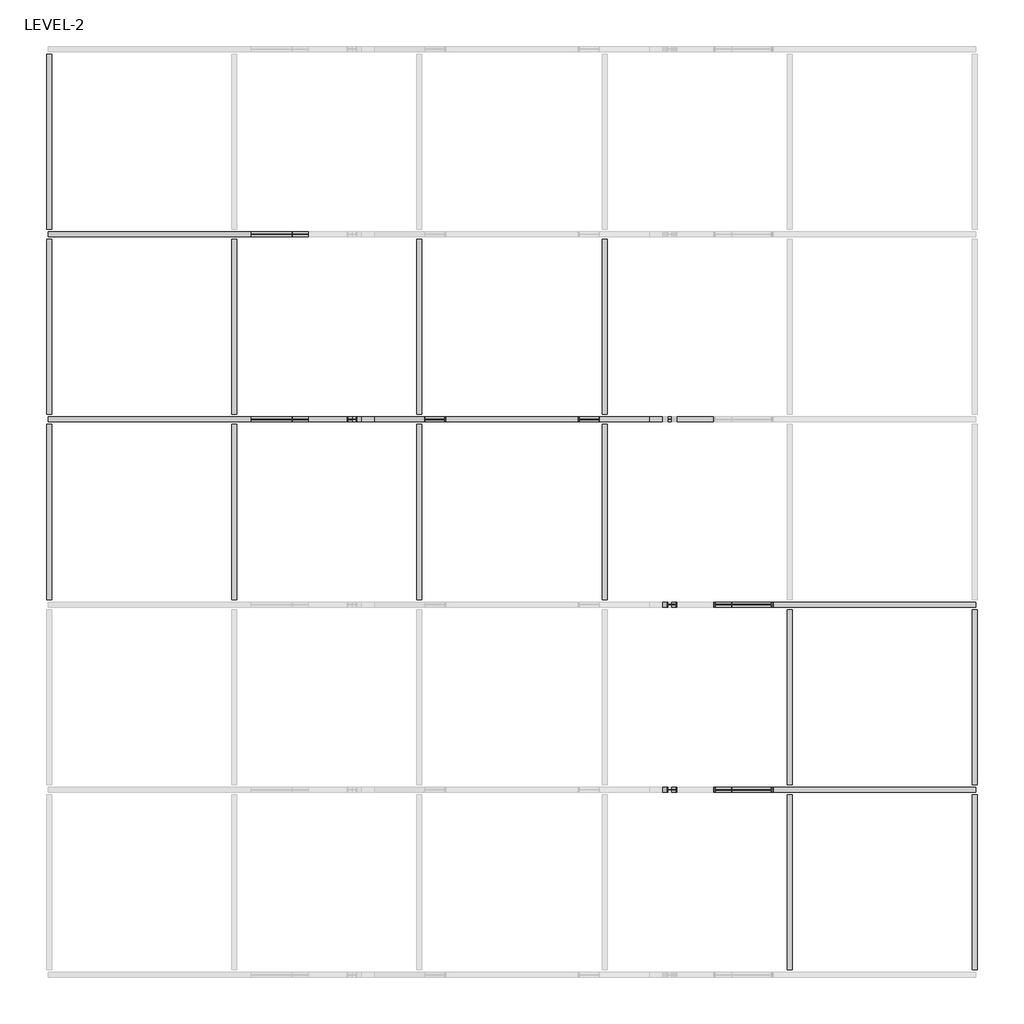
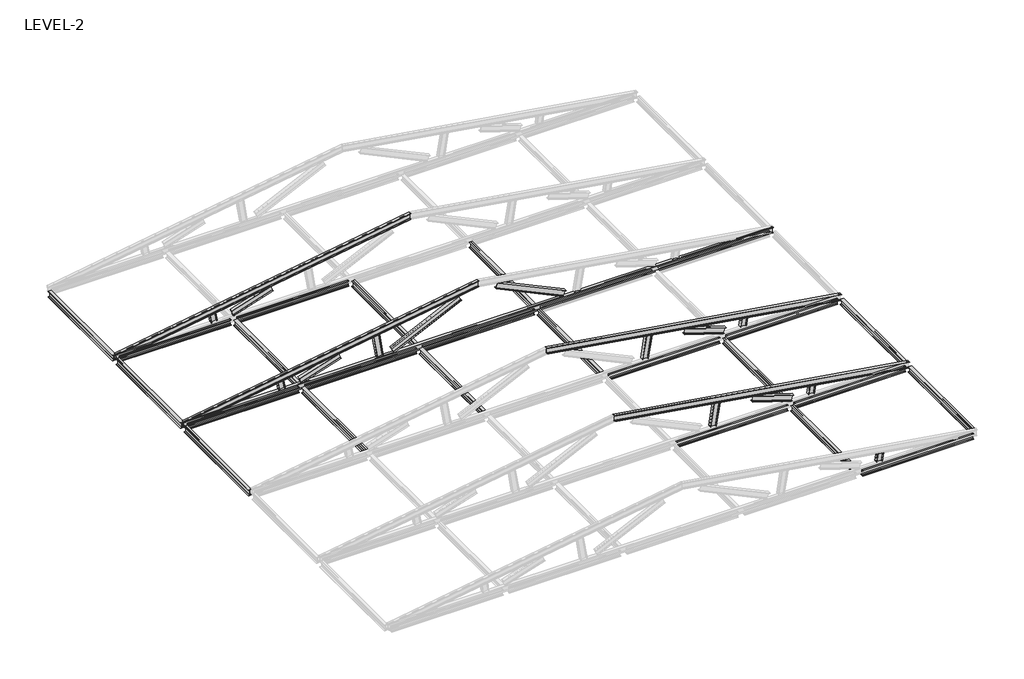
# One storey, part 2 of 3: 42 beams.
"""IFC4 building model written with IfcOpenShell, lengths in millimetres."""

from ifc_helpers import new_model, si_unit, frame, origin, place, context, project, spatial, polyline, circle_curve, ellipse_curve, transform, mapped, element, save
from ifc_brep_helpers import plane_surface, revolved_surface, advanced_brep
from components import ub_universal_beams_ub305x165x40_616d6e4e, ub_universal_beams_ub305x165x40_3f70edd5, ub_universal_beams_ub305x165x40_c9eec61f, ub_universal_beams_ub305x165x40_c956ba20, ub_universal_beams_ub305x165x40_f58164a9, ub_universal_beams_ub305x165x40_ef0a91e2, ub_universal_beams_ub305x165x40_83ed4f69, ub_universal_beams_ub305x165x40_46a3dc55, ub_universal_beams_ub305x165x40_0b6a72e4, ub_universal_beams_ub305x165x40_63d5ebb1, ub_universal_beams_ub305x165x40_05d28e63

model = new_model("IFC4")

# Units and contexts
model_context = context("Model", 3, world=origin())
ifc_project = project(units=[si_unit("LENGTHUNIT", "METRE", prefix="MILLI")], contexts=[model_context])

# Site, building, storey
site = spatial("IfcSite", under=ifc_project)
building = spatial("IfcBuilding", under=site)
storey = spatial("IfcBuildingStorey", under=building, Name="LEVEL-2", Elevation=4267.0)

# Beams
placement = place(None, origin())
element("IfcBeam", 1, ObjectType="UB-Universal Beams : UB305x165x40", at=placement, inside=storey, context=model_context, shape_type="AdvancedBrep", body=[
    advanced_brep(
    [(11917.6451312, -8149.9765895, 4127.2241081), (11917.6451312, -8220.5765895, 4127.2241081), (11919.0296431, -8229.4765895, 4136.0157591), (11960.2849884, -8229.4765895, 4397.9872012), (11961.6695003, -8220.5765895, 4406.7788522), (11961.6695003, -8149.9765895, 4406.7788522), (11963.2562444, -8149.9765895, 4416.8546768), (11963.2562444, -8314.9765895, 4416.8546768), (11961.6695003, -8314.9765895, 4406.7788522), (11961.6695003, -8244.3765895, 4406.7788522), (11960.2849884, -8235.4765895, 4397.9872012), (11919.0296431, -8235.4765895, 4136.0157591), (11917.6451312, -8244.3765895, 4127.2241081), (11917.6451312, -8314.9765895, 4127.2241081), (11916.0583871, -8314.9765895, 4117.1482834), (11916.0583871, -8149.9765895, 4117.1482834), (-3300.3332854, -8149.9765895, 6523.7561422), (-3300.3332854, -8220.5765895, 6523.7561422), (-3300.3332854, -8229.4765895, 6532.7658266), (-3300.3332854, -8229.4765895, 6801.2341734), (-3300.3332854, -8220.5765895, 6810.2438578), (-3300.3332854, -8149.9765895, 6810.2438578), (-3300.3332854, -8149.9765895, 6820.5695634), (-3300.3332854, -8314.9765895, 6820.5695634), (-3300.3332854, -8314.9765895, 6810.2438578), (-3300.3332854, -8244.3765895, 6810.2438578), (-3300.3332854, -8235.4765895, 6801.2341734), (-3300.3332854, -8235.4765895, 6532.7658266), (-3300.3332854, -8244.3765895, 6523.7561422), (-3300.3332854, -8314.9765895, 6523.7561422), (-3300.3332854, -8314.9765895, 6513.4304366), (-3300.3332854, -8149.9765895, 6513.4304366)],
    [
        (0, 1),
        (1, 2, circle_curve(frame((11919.0296431, -8220.5765895, 4136.0157591), z_axis=(-0.9878259507117182, 0.0, 0.1555631418443652), x_axis=(0.0, -1.0, 0.0)), 8.9)),
        (2, 3),
        (3, 4, circle_curve(frame((11960.2849884, -8220.5765895, 4397.9872012), z_axis=(-0.9878259507117182, 0.0, 0.1555631418443652), x_axis=(0.0, -1.0, 0.0)), 8.9)),
        (4, 5),
        (5, 6),
        (6, 7),
        (7, 8),
        (8, 9),
        (9, 10, circle_curve(frame((11960.2849884, -8244.3765895, 4397.9872012), z_axis=(-0.9878259507117182, 0.0, 0.1555631418443652), x_axis=(0.0, -1.0, 0.0)), 8.9)),
        (10, 11),
        (11, 12, circle_curve(frame((11919.0296431, -8244.3765895, 4136.0157591), z_axis=(-0.9878259507117182, 0.0, 0.1555631418443652), x_axis=(0.0, -1.0, 0.0)), 8.9)),
        (12, 13),
        (13, 14),
        (14, 15),
        (15, 0),
        (0, 16),
        (16, 17),
        (17, 1),
        (17, 18, ellipse_curve(frame((-3300.3332854, -8220.5765895, 6532.7658266), z_axis=(-1.0, 0.0, 0.0), x_axis=(0.0, 0.0, 1.0)), 9.0096843, 8.9)),
        (18, 2),
        (18, 19),
        (19, 3),
        (19, 20, ellipse_curve(frame((-3300.3332854, -8220.5765895, 6801.2341734), z_axis=(-1.0, 0.0, 0.0), x_axis=(0.0, 0.0, 1.0)), 9.0096843, 8.9)),
        (20, 4),
        (20, 21),
        (21, 5),
        (21, 22),
        (22, 6),
        (22, 23),
        (23, 7),
        (23, 24),
        (24, 8),
        (24, 25),
        (25, 9),
        (25, 26, ellipse_curve(frame((-3300.3332854, -8244.3765895, 6801.2341734), z_axis=(-1.0, 0.0, 0.0), x_axis=(0.0, 0.0, 1.0)), 9.0096843, 8.9)),
        (26, 10),
        (26, 27),
        (27, 11),
        (27, 28, ellipse_curve(frame((-3300.3332854, -8244.3765895, 6532.7658266), z_axis=(-1.0, 0.0, 0.0), x_axis=(0.0, 0.0, 1.0)), 9.0096843, 8.9)),
        (28, 12),
        (28, 29),
        (29, 13),
        (29, 30),
        (30, 14),
        (30, 31),
        (31, 15),
        (31, 16),
    ],
    [
        plane_surface(frame((11939.6573157, -8232.4765895, 4267.0014801), z_axis=(0.9878259507117182, 0.0, -0.1555631418443652), x_axis=(0.1555631418443652, 0.0, 0.9878259507117182))),
        plane_surface(frame((11917.6451312, -8149.9765895, 4127.2241081), z_axis=(0.1555631418443652, 0.0, 0.9878259507117182), x_axis=(-0.9878259507117182, 0.0, 0.1555631418443652))),
        revolved_surface(polyline([(-3301.7177973591024, -8229.4765895, 6532.983859959702), (11919.029643166847, -8229.4765895, 4136.015759089472)]), (11919.0296431, -8220.5765895, 4136.0157591), (-0.9878259507117182, 0.0, 0.1555631418443652)),
        plane_surface(frame((11919.0296431, -8229.4765895, 4136.0157591), z_axis=(0.0, 1.0, 0.0), x_axis=(-0.9878259507117182, 0.0, 0.1555631418443652))),
        revolved_surface(polyline([(-3301.717797363457, -8229.4765895, 6801.452206832042), (11960.2849884, -8229.4765895, 4397.9872012)]), (11960.2849884, -8220.5765895, 4397.9872012), (-0.9878259507117182, 0.0, 0.1555631418443652)),
        plane_surface(frame((11961.6695003, -8220.5765895, 4406.7788522), z_axis=(-0.1555631418443652, 0.0, -0.9878259507117182), x_axis=(-0.9878259507117182, 0.0, 0.1555631418443652))),
        plane_surface(frame((11961.6695003, -8149.9765895, 4406.7788522), z_axis=(0.0, 1.0, 0.0), x_axis=(-0.9878259507117182, 0.0, 0.1555631418443652))),
        plane_surface(frame((11963.2562444, -8149.9765895, 4416.8546768), z_axis=(0.1555631418443652, 0.0, 0.9878259507117182), x_axis=(-0.9878259507117182, 0.0, 0.1555631418443652))),
        plane_surface(frame((11963.2562444, -8314.9765895, 4416.8546768), z_axis=(0.0, -1.0, 0.0), x_axis=(-0.9878259507117182, 0.0, 0.1555631418443652))),
        plane_surface(frame((11961.6695003, -8314.9765895, 4406.7788522), z_axis=(-0.1555631418443652, 0.0, -0.9878259507117182), x_axis=(-0.9878259507117182, 0.0, 0.1555631418443652))),
        revolved_surface(polyline([(-3301.717797363457, -8253.2765895, 6801.452206832042), (11960.2849884, -8253.2765895, 4397.9872012)]), (11960.2849884, -8244.3765895, 4397.9872012), (-0.9878259507117182, 0.0, 0.1555631418443652)),
        plane_surface(frame((11960.2849884, -8235.4765895, 4397.9872012), z_axis=(0.0, -1.0, 0.0), x_axis=(-0.9878259507117182, 0.0, 0.1555631418443652))),
        revolved_surface(polyline([(-3301.7177973591024, -8253.2765895, 6532.983859959702), (11919.029643166847, -8253.2765895, 4136.015759089472)]), (11919.0296431, -8244.3765895, 4136.0157591), (-0.9878259507117182, 0.0, 0.1555631418443652)),
        plane_surface(frame((11917.6451312, -8244.3765895, 4127.2241081), z_axis=(0.1555631418443652, 0.0, 0.9878259507117182), x_axis=(-0.9878259507117182, 0.0, 0.1555631418443652))),
        plane_surface(frame((11917.6451312, -8314.9765895, 4127.2241081), z_axis=(0.0, -1.0, 0.0), x_axis=(-0.9878259507117182, 0.0, 0.1555631418443652))),
        plane_surface(frame((11916.0583871, -8314.9765895, 4117.1482834), z_axis=(-0.1555631418443652, 0.0, -0.9878259507117182), x_axis=(-0.9878259507117182, 0.0, 0.1555631418443652))),
        plane_surface(frame((11916.0583871, -8149.9765895, 4117.1482834), z_axis=(0.0, 1.0, 0.0), x_axis=(-0.9878259507117182, 0.0, 0.1555631418443652))),
        plane_surface(frame((-3300.3332854, -8232.4765895, 6820.5695634), z_axis=(-1.0, 0.0, 0.0), x_axis=(0.0, 1.0, 0.0))),
    ],
    [
        (0, [[1, 2, 3, 4, 5, 6, 7, 8, 9, 10, 11, 12, 13, 14, 15, 16]]),
        (1, [[-1, 17, 18, 19]]),
        (2, [[-2, -19, 20, 21]]),
        (3, [[-3, -21, 22, 23]]),
        (4, [[-4, -23, 24, 25]]),
        (5, [[-5, -25, 26, 27]]),
        (6, [[-6, -27, 28, 29]]),
        (7, [[-7, -29, 30, 31]]),
        (8, [[-8, -31, 32, 33]]),
        (9, [[-9, -33, 34, 35]]),
        (10, [[-10, -35, 36, 37]]),
        (11, [[-11, -37, 38, 39]]),
        (12, [[-12, -39, 40, 41]]),
        (13, [[-13, -41, 42, 43]]),
        (14, [[-14, -43, 44, 45]]),
        (15, [[-15, -45, 46, 47]]),
        (16, [[-16, -47, 48, -17]]),
        (17, [[-48, -46, -44, -42, -40, -38, -36, -34, -32, -30, -28, -26, -24, -22, -20, -18]]),
    ],
),
])
element("IfcBeam", 2, ObjectType="UB-Universal Beams : UB305x165x40", at=placement, inside=storey, context=model_context, shape_type="AdvancedBrep", body=[
    advanced_brep(
    [(11917.6451312, -2053.9765895, 4127.2241081), (11917.6451312, -2124.5765895, 4127.2241081), (11919.0296431, -2133.4765895, 4136.0157591), (11960.2849884, -2133.4765895, 4397.9872012), (11961.6695003, -2124.5765895, 4406.7788522), (11961.6695003, -2053.9765895, 4406.7788522), (11963.2562444, -2053.9765895, 4416.8546768), (11963.2562444, -2218.9765895, 4416.8546768), (11961.6695003, -2218.9765895, 4406.7788522), (11961.6695003, -2148.3765895, 4406.7788522), (11960.2849884, -2139.4765895, 4397.9872012), (11919.0296431, -2139.4765895, 4136.0157591), (11917.6451312, -2148.3765895, 4127.2241081), (11917.6451312, -2218.9765895, 4127.2241081), (11916.0583871, -2218.9765895, 4117.1482834), (11916.0583871, -2053.9765895, 4117.1482834), (-3300.3332854, -2053.9765895, 6523.7561422), (-3300.3332854, -2124.5765895, 6523.7561422), (-3300.3332854, -2133.4765895, 6532.7658266), (-3300.3332854, -2133.4765895, 6801.2341734), (-3300.3332854, -2124.5765895, 6810.2438578), (-3300.3332854, -2053.9765895, 6810.2438578), (-3300.3332854, -2053.9765895, 6820.5695634), (-3300.3332854, -2218.9765895, 6820.5695634), (-3300.3332854, -2218.9765895, 6810.2438578), (-3300.3332854, -2148.3765895, 6810.2438578), (-3300.3332854, -2139.4765895, 6801.2341734), (-3300.3332854, -2139.4765895, 6532.7658266), (-3300.3332854, -2148.3765895, 6523.7561422), (-3300.3332854, -2218.9765895, 6523.7561422), (-3300.3332854, -2218.9765895, 6513.4304366), (-3300.3332854, -2053.9765895, 6513.4304366)],
    [
        (0, 1),
        (1, 2, circle_curve(frame((11919.0296431, -2124.5765895, 4136.0157591), z_axis=(-0.9878259507117182, 0.0, 0.1555631418443652), x_axis=(0.0, -1.0, 0.0)), 8.9)),
        (2, 3),
        (3, 4, circle_curve(frame((11960.2849884, -2124.5765895, 4397.9872012), z_axis=(-0.9878259507117182, 0.0, 0.1555631418443652), x_axis=(0.0, -1.0, 0.0)), 8.9)),
        (4, 5),
        (5, 6),
        (6, 7),
        (7, 8),
        (8, 9),
        (9, 10, circle_curve(frame((11960.2849884, -2148.3765895, 4397.9872012), z_axis=(-0.9878259507117182, 0.0, 0.1555631418443652), x_axis=(0.0, -1.0, 0.0)), 8.9)),
        (10, 11),
        (11, 12, circle_curve(frame((11919.0296431, -2148.3765895, 4136.0157591), z_axis=(-0.9878259507117182, 0.0, 0.1555631418443652), x_axis=(0.0, -1.0, 0.0)), 8.9)),
        (12, 13),
        (13, 14),
        (14, 15),
        (15, 0),
        (0, 16),
        (16, 17),
        (17, 1),
        (17, 18, ellipse_curve(frame((-3300.3332854, -2124.5765895, 6532.7658266), z_axis=(-1.0, 0.0, 0.0), x_axis=(0.0, 0.0, 1.0)), 9.0096843, 8.9)),
        (18, 2),
        (18, 19),
        (19, 3),
        (19, 20, ellipse_curve(frame((-3300.3332854, -2124.5765895, 6801.2341734), z_axis=(-1.0, 0.0, 0.0), x_axis=(0.0, 0.0, 1.0)), 9.0096843, 8.9)),
        (20, 4),
        (20, 21),
        (21, 5),
        (21, 22),
        (22, 6),
        (22, 23),
        (23, 7),
        (23, 24),
        (24, 8),
        (24, 25),
        (25, 9),
        (25, 26, ellipse_curve(frame((-3300.3332854, -2148.3765895, 6801.2341734), z_axis=(-1.0, 0.0, 0.0), x_axis=(0.0, 0.0, 1.0)), 9.0096843, 8.9)),
        (26, 10),
        (26, 27),
        (27, 11),
        (27, 28, ellipse_curve(frame((-3300.3332854, -2148.3765895, 6532.7658266), z_axis=(-1.0, 0.0, 0.0), x_axis=(0.0, 0.0, 1.0)), 9.0096843, 8.9)),
        (28, 12),
        (28, 29),
        (29, 13),
        (29, 30),
        (30, 14),
        (30, 31),
        (31, 15),
        (31, 16),
    ],
    [
        plane_surface(frame((11939.6573157, -2136.4765895, 4267.0014801), z_axis=(0.9878259507117182, 0.0, -0.1555631418443652), x_axis=(0.1555631418443652, 0.0, 0.9878259507117182))),
        plane_surface(frame((11917.6451312, -2053.9765895, 4127.2241081), z_axis=(0.1555631418443652, 0.0, 0.9878259507117182), x_axis=(-0.9878259507117182, 0.0, 0.1555631418443652))),
        revolved_surface(polyline([(-3301.7177973591024, -2133.4765895, 6532.983859959702), (11919.029643166847, -2133.4765895, 4136.015759089472)]), (11919.0296431, -2124.5765895, 4136.0157591), (-0.9878259507117182, 0.0, 0.1555631418443652)),
        plane_surface(frame((11919.0296431, -2133.4765895, 4136.0157591), z_axis=(0.0, 1.0, 0.0), x_axis=(-0.9878259507117182, 0.0, 0.1555631418443652))),
        revolved_surface(polyline([(-3301.717797363457, -2133.4765895, 6801.452206832042), (11960.2849884, -2133.4765895, 4397.9872012)]), (11960.2849884, -2124.5765895, 4397.9872012), (-0.9878259507117182, 0.0, 0.1555631418443652)),
        plane_surface(frame((11961.6695003, -2124.5765895, 4406.7788522), z_axis=(-0.1555631418443652, 0.0, -0.9878259507117182), x_axis=(-0.9878259507117182, 0.0, 0.1555631418443652))),
        plane_surface(frame((11961.6695003, -2053.9765895, 4406.7788522), z_axis=(0.0, 1.0, 0.0), x_axis=(-0.9878259507117182, 0.0, 0.1555631418443652))),
        plane_surface(frame((11963.2562444, -2053.9765895, 4416.8546768), z_axis=(0.1555631418443652, 0.0, 0.9878259507117182), x_axis=(-0.9878259507117182, 0.0, 0.1555631418443652))),
        plane_surface(frame((11963.2562444, -2218.9765895, 4416.8546768), z_axis=(0.0, -1.0, 0.0), x_axis=(-0.9878259507117182, 0.0, 0.1555631418443652))),
        plane_surface(frame((11961.6695003, -2218.9765895, 4406.7788522), z_axis=(-0.1555631418443652, 0.0, -0.9878259507117182), x_axis=(-0.9878259507117182, 0.0, 0.1555631418443652))),
        revolved_surface(polyline([(-3301.717797363457, -2157.2765895000002, 6801.452206832042), (11960.2849884, -2157.2765895000002, 4397.9872012)]), (11960.2849884, -2148.3765895, 4397.9872012), (-0.9878259507117182, 0.0, 0.1555631418443652)),
        plane_surface(frame((11960.2849884, -2139.4765895, 4397.9872012), z_axis=(0.0, -1.0, 0.0), x_axis=(-0.9878259507117182, 0.0, 0.1555631418443652))),
        revolved_surface(polyline([(-3301.7177973591024, -2157.2765895000002, 6532.983859959702), (11919.029643166847, -2157.2765895000002, 4136.015759089472)]), (11919.0296431, -2148.3765895, 4136.0157591), (-0.9878259507117182, 0.0, 0.1555631418443652)),
        plane_surface(frame((11917.6451312, -2148.3765895, 4127.2241081), z_axis=(0.1555631418443652, 0.0, 0.9878259507117182), x_axis=(-0.9878259507117182, 0.0, 0.1555631418443652))),
        plane_surface(frame((11917.6451312, -2218.9765895, 4127.2241081), z_axis=(0.0, -1.0, 0.0), x_axis=(-0.9878259507117182, 0.0, 0.1555631418443652))),
        plane_surface(frame((11916.0583871, -2218.9765895, 4117.1482834), z_axis=(-0.1555631418443652, 0.0, -0.9878259507117182), x_axis=(-0.9878259507117182, 0.0, 0.1555631418443652))),
        plane_surface(frame((11916.0583871, -2053.9765895, 4117.1482834), z_axis=(0.0, 1.0, 0.0), x_axis=(-0.9878259507117182, 0.0, 0.1555631418443652))),
        plane_surface(frame((-3300.3332854, -2136.4765895, 6820.5695634), z_axis=(-1.0, 0.0, 0.0), x_axis=(0.0, 1.0, 0.0))),
    ],
    [
        (0, [[1, 2, 3, 4, 5, 6, 7, 8, 9, 10, 11, 12, 13, 14, 15, 16]]),
        (1, [[-1, 17, 18, 19]]),
        (2, [[-2, -19, 20, 21]]),
        (3, [[-3, -21, 22, 23]]),
        (4, [[-4, -23, 24, 25]]),
        (5, [[-5, -25, 26, 27]]),
        (6, [[-6, -27, 28, 29]]),
        (7, [[-7, -29, 30, 31]]),
        (8, [[-8, -31, 32, 33]]),
        (9, [[-9, -33, 34, 35]]),
        (10, [[-10, -35, 36, 37]]),
        (11, [[-11, -37, 38, 39]]),
        (12, [[-12, -39, 40, 41]]),
        (13, [[-13, -41, 42, 43]]),
        (14, [[-14, -43, 44, 45]]),
        (15, [[-15, -45, 46, 47]]),
        (16, [[-16, -47, 48, -17]]),
        (17, [[-48, -46, -44, -42, -40, -38, -36, -34, -32, -30, -28, -26, -24, -22, -20, -18]]),
    ],
),
])
element("IfcBeam", 3, ObjectType="UB-Universal Beams : UB305x165x40", at=placement, inside=storey, context=model_context, shape_type="AdvancedBrep", body=[
    advanced_brep(
    [(-18518.3117021, 4042.0234105, 4127.2241081), (-18516.724958, 4042.0234105, 4117.1482834), (-18516.724958, 3877.0234105, 4117.1482834), (-18518.3117021, 3877.0234105, 4127.2241081), (-18518.3117021, 3947.6234105, 4127.2241081), (-18519.696214, 3956.5234105, 4136.0157591), (-18560.9515593, 3956.5234105, 4397.9872012), (-18562.3360712, 3947.6234105, 4406.7788522), (-18562.3360712, 3877.0234105, 4406.7788522), (-18563.9228153, 3877.0234105, 4416.8546768), (-18563.9228153, 4042.0234105, 4416.8546768), (-18562.3360712, 4042.0234105, 4406.7788522), (-18562.3360712, 3971.4234105, 4406.7788522), (-18560.9515593, 3962.5234105, 4397.9872012), (-18519.696214, 3962.5234105, 4136.0157591), (-18518.3117021, 3971.4234105, 4127.2241081), (-3300.3332854, 3971.4234105, 6523.7561422), (-3300.3332854, 4042.0234105, 6523.7561422), (-3300.3332854, 3962.5234105, 6532.7658266), (-3300.3332854, 3962.5234105, 6801.2341734), (-3300.3332854, 3971.4234105, 6810.2438578), (-3300.3332854, 4042.0234105, 6810.2438578), (-3300.3332854, 4042.0234105, 6820.5695634), (-3300.3332854, 3877.0234105, 6820.5695634), (-3300.3332854, 3877.0234105, 6810.2438578), (-3300.3332854, 3947.6234105, 6810.2438578), (-3300.3332854, 3956.5234105, 6801.2341734), (-3300.3332854, 3956.5234105, 6532.7658266), (-3300.3332854, 3947.6234105, 6523.7561422), (-3300.3332854, 3877.0234105, 6523.7561422), (-3300.3332854, 3877.0234105, 6513.4304366), (-3300.3332854, 4042.0234105, 6513.4304366)],
    [
        (0, 1),
        (1, 2),
        (2, 3),
        (3, 4),
        (4, 5, circle_curve(frame((-18519.696214, 3947.6234105, 4136.0157591), z_axis=(0.9878259507117182, 0.0, 0.1555631418443652), x_axis=(0.0, -1.0, 0.0)), 8.9)),
        (5, 6),
        (6, 7, circle_curve(frame((-18560.9515593, 3947.6234105, 4397.9872012), z_axis=(0.9878259507117182, 0.0, 0.1555631418443652), x_axis=(0.0, -1.0, 0.0)), 8.9)),
        (7, 8),
        (8, 9),
        (9, 10),
        (10, 11),
        (11, 12),
        (12, 13, circle_curve(frame((-18560.9515593, 3971.4234105, 4397.9872012), z_axis=(0.9878259507117182, 0.0, 0.1555631418443652), x_axis=(0.0, -1.0, 0.0)), 8.9)),
        (13, 14),
        (14, 15, circle_curve(frame((-18519.696214, 3971.4234105, 4136.0157591), z_axis=(0.9878259507117182, 0.0, 0.1555631418443652), x_axis=(0.0, -1.0, 0.0)), 8.9)),
        (15, 0),
        (16, 17),
        (17, 0),
        (15, 16),
        (18, 16, ellipse_curve(frame((-3300.3332854, 3971.4234105, 6532.7658266), z_axis=(1.0, 0.0, 0.0), x_axis=(0.0, 0.0, -1.0)), 9.0096843, 8.9)),
        (14, 18),
        (19, 18),
        (13, 19),
        (20, 19, ellipse_curve(frame((-3300.3332854, 3971.4234105, 6801.2341734), z_axis=(1.0, 0.0, 0.0), x_axis=(0.0, 0.0, -1.0)), 9.0096843, 8.9)),
        (12, 20),
        (21, 20),
        (11, 21),
        (22, 21),
        (10, 22),
        (23, 22),
        (9, 23),
        (24, 23),
        (8, 24),
        (25, 24),
        (7, 25),
        (26, 25, ellipse_curve(frame((-3300.3332854, 3947.6234105, 6801.2341734), z_axis=(1.0, 0.0, 0.0), x_axis=(0.0, 0.0, -1.0)), 9.0096843, 8.9)),
        (6, 26),
        (27, 26),
        (5, 27),
        (28, 27, ellipse_curve(frame((-3300.3332854, 3947.6234105, 6532.7658266), z_axis=(1.0, 0.0, 0.0), x_axis=(0.0, 0.0, -1.0)), 9.0096843, 8.9)),
        (4, 28),
        (29, 28),
        (3, 29),
        (30, 29),
        (2, 30),
        (31, 30),
        (1, 31),
        (17, 31),
    ],
    [
        plane_surface(frame((-18540.3238866, 3959.5234105, 4267.0014801), z_axis=(-0.9878259507117182, 0.0, -0.1555631418443652), x_axis=(-0.1555631418443652, 0.0, 0.9878259507117182))),
        plane_surface(frame((-3278.3304997, 4042.0234105, 6527.2211478), z_axis=(-0.1555631418443652, 0.0, 0.9878259507117182), x_axis=(-0.9878259507117182, 0.0, -0.1555631418443652))),
        revolved_surface(polyline([(-18519.696214059466, 3962.5234105, 4136.015759042602), (-3298.948773435937, 3962.5234105, 6532.983859928199)]), (-3279.7150116, 3971.4234105, 6536.0127988), (-0.9878259507117182, 0.0, -0.1555631418443652)),
        plane_surface(frame((-3279.7150116, 3962.5234105, 6536.0127988), z_axis=(0.0, 1.0, 0.0), x_axis=(-0.9878259507117182, 0.0, -0.1555631418443652))),
        revolved_surface(polyline([(-18560.95155929262, 3962.5234105, 4397.98720115313), (-3298.948773431581, 3962.5234105, 6801.452206800539)]), (-3320.9703569, 3971.4234105, 6797.9842409), (-0.9878259507117182, 0.0, -0.1555631418443652)),
        plane_surface(frame((-3322.3548688, 3971.4234105, 6806.7758919), z_axis=(0.1555631418443652, 0.0, -0.9878259507117182), x_axis=(-0.9878259507117182, 0.0, -0.1555631418443652))),
        plane_surface(frame((-3322.3548688, 4042.0234105, 6806.7758919), z_axis=(0.0, 1.0, 0.0), x_axis=(-0.9878259507117182, 0.0, -0.1555631418443652))),
        plane_surface(frame((-3323.9416129, 4042.0234105, 6816.8517166), z_axis=(-0.1555631418443652, 0.0, 0.9878259507117182), x_axis=(-0.9878259507117182, 0.0, -0.1555631418443652))),
        plane_surface(frame((-3323.9416129, 3877.0234105, 6816.8517166), z_axis=(0.0, -1.0, 0.0), x_axis=(-0.9878259507117182, 0.0, -0.1555631418443652))),
        plane_surface(frame((-3322.3548688, 3877.0234105, 6806.7758919), z_axis=(0.1555631418443652, 0.0, -0.9878259507117182), x_axis=(-0.9878259507117182, 0.0, -0.1555631418443652))),
        revolved_surface(polyline([(-18560.95155929262, 3938.7234104999998, 4397.98720115313), (-3298.948773431581, 3938.7234104999998, 6801.452206800539)]), (-3320.9703569, 3947.6234105, 6797.9842409), (-0.9878259507117182, 0.0, -0.1555631418443652)),
        plane_surface(frame((-3320.9703569, 3956.5234105, 6797.9842409), z_axis=(0.0, -1.0, 0.0), x_axis=(-0.9878259507117182, 0.0, -0.1555631418443652))),
        revolved_surface(polyline([(-18519.696214059466, 3938.7234104999998, 4136.015759042602), (-3298.948773435937, 3938.7234104999998, 6532.983859928199)]), (-3279.7150116, 3947.6234105, 6536.0127988), (-0.9878259507117182, 0.0, -0.1555631418443652)),
        plane_surface(frame((-3278.3304997, 3947.6234105, 6527.2211478), z_axis=(-0.1555631418443652, 0.0, 0.9878259507117182), x_axis=(-0.9878259507117182, 0.0, -0.1555631418443652))),
        plane_surface(frame((-3278.3304997, 3877.0234105, 6527.2211478), z_axis=(0.0, -1.0, 0.0), x_axis=(-0.9878259507117182, 0.0, -0.1555631418443652))),
        plane_surface(frame((-3276.7437556, 3877.0234105, 6517.1453232), z_axis=(0.1555631418443652, 0.0, -0.9878259507117182), x_axis=(-0.9878259507117182, 0.0, -0.1555631418443652))),
        plane_surface(frame((-3276.7437556, 4042.0234105, 6517.1453232), z_axis=(0.0, 1.0, 0.0), x_axis=(-0.9878259507117182, 0.0, -0.1555631418443652))),
        plane_surface(frame((-3300.3332854, 3959.5234105, 6820.5695634), z_axis=(1.0, 0.0, 0.0), x_axis=(0.0, -1.0, 0.0))),
    ],
    [
        (0, [[1, 2, 3, 4, 5, 6, 7, 8, 9, 10, 11, 12, 13, 14, 15, 16]]),
        (1, [[17, 18, -16, 19]]),
        (2, [[20, -19, -15, 21]]),
        (3, [[22, -21, -14, 23]]),
        (4, [[24, -23, -13, 25]]),
        (5, [[26, -25, -12, 27]]),
        (6, [[28, -27, -11, 29]]),
        (7, [[30, -29, -10, 31]]),
        (8, [[32, -31, -9, 33]]),
        (9, [[34, -33, -8, 35]]),
        (10, [[36, -35, -7, 37]]),
        (11, [[38, -37, -6, 39]]),
        (12, [[40, -39, -5, 41]]),
        (13, [[42, -41, -4, 43]]),
        (14, [[44, -43, -3, 45]]),
        (15, [[46, -45, -2, 47]]),
        (16, [[48, -47, -1, -18]]),
        (17, [[-17, -20, -22, -24, -26, -28, -30, -32, -34, -36, -38, -40, -42, -44, -46, -48]]),
    ],
),
])
element("IfcBeam", 4, ObjectType="UB-Universal Beams : UB305x165x40", at=placement, inside=storey, context=model_context, shape_type="AdvancedBrep", body=[
    advanced_brep(
    [(-18518.3117021, 10138.0234105, 4127.2241081), (-18516.724958, 10138.0234105, 4117.1482834), (-18516.724958, 9973.0234105, 4117.1482834), (-18518.3117021, 9973.0234105, 4127.2241081), (-18518.3117021, 10043.6234105, 4127.2241081), (-18519.696214, 10052.5234105, 4136.0157591), (-18560.9515593, 10052.5234105, 4397.9872012), (-18562.3360712, 10043.6234105, 4406.7788522), (-18562.3360712, 9973.0234105, 4406.7788522), (-18563.9228153, 9973.0234105, 4416.8546768), (-18563.9228153, 10138.0234105, 4416.8546768), (-18562.3360712, 10138.0234105, 4406.7788522), (-18562.3360712, 10067.4234105, 4406.7788522), (-18560.9515593, 10058.5234105, 4397.9872012), (-18519.696214, 10058.5234105, 4136.0157591), (-18518.3117021, 10067.4234105, 4127.2241081), (-3300.3332854, 10067.4234105, 6523.7561422), (-3300.3332854, 10138.0234105, 6523.7561422), (-3300.3332854, 10058.5234105, 6532.7658266), (-3300.3332854, 10058.5234105, 6801.2341734), (-3300.3332854, 10067.4234105, 6810.2438578), (-3300.3332854, 10138.0234105, 6810.2438578), (-3300.3332854, 10138.0234105, 6820.5695634), (-3300.3332854, 9973.0234105, 6820.5695634), (-3300.3332854, 9973.0234105, 6810.2438578), (-3300.3332854, 10043.6234105, 6810.2438578), (-3300.3332854, 10052.5234105, 6801.2341734), (-3300.3332854, 10052.5234105, 6532.7658266), (-3300.3332854, 10043.6234105, 6523.7561422), (-3300.3332854, 9973.0234105, 6523.7561422), (-3300.3332854, 9973.0234105, 6513.4304366), (-3300.3332854, 10138.0234105, 6513.4304366)],
    [
        (0, 1),
        (1, 2),
        (2, 3),
        (3, 4),
        (4, 5, circle_curve(frame((-18519.696214, 10043.6234105, 4136.0157591), z_axis=(0.9878259507117182, 0.0, 0.1555631418443652), x_axis=(0.0, -1.0, 0.0)), 8.9)),
        (5, 6),
        (6, 7, circle_curve(frame((-18560.9515593, 10043.6234105, 4397.9872012), z_axis=(0.9878259507117182, 0.0, 0.1555631418443652), x_axis=(0.0, -1.0, 0.0)), 8.9)),
        (7, 8),
        (8, 9),
        (9, 10),
        (10, 11),
        (11, 12),
        (12, 13, circle_curve(frame((-18560.9515593, 10067.4234105, 4397.9872012), z_axis=(0.9878259507117182, 0.0, 0.1555631418443652), x_axis=(0.0, -1.0, 0.0)), 8.9)),
        (13, 14),
        (14, 15, circle_curve(frame((-18519.696214, 10067.4234105, 4136.0157591), z_axis=(0.9878259507117182, 0.0, 0.1555631418443652), x_axis=(0.0, -1.0, 0.0)), 8.9)),
        (15, 0),
        (16, 17),
        (17, 0),
        (15, 16),
        (18, 16, ellipse_curve(frame((-3300.3332854, 10067.4234105, 6532.7658266), z_axis=(1.0, 0.0, 0.0), x_axis=(0.0, 0.0, -1.0)), 9.0096843, 8.9)),
        (14, 18),
        (19, 18),
        (13, 19),
        (20, 19, ellipse_curve(frame((-3300.3332854, 10067.4234105, 6801.2341734), z_axis=(1.0, 0.0, 0.0), x_axis=(0.0, 0.0, -1.0)), 9.0096843, 8.9)),
        (12, 20),
        (21, 20),
        (11, 21),
        (22, 21),
        (10, 22),
        (23, 22),
        (9, 23),
        (24, 23),
        (8, 24),
        (25, 24),
        (7, 25),
        (26, 25, ellipse_curve(frame((-3300.3332854, 10043.6234105, 6801.2341734), z_axis=(1.0, 0.0, 0.0), x_axis=(0.0, 0.0, -1.0)), 9.0096843, 8.9)),
        (6, 26),
        (27, 26),
        (5, 27),
        (28, 27, ellipse_curve(frame((-3300.3332854, 10043.6234105, 6532.7658266), z_axis=(1.0, 0.0, 0.0), x_axis=(0.0, 0.0, -1.0)), 9.0096843, 8.9)),
        (4, 28),
        (29, 28),
        (3, 29),
        (30, 29),
        (2, 30),
        (31, 30),
        (1, 31),
        (17, 31),
    ],
    [
        plane_surface(frame((-18540.3238866, 10055.5234105, 4267.0014801), z_axis=(-0.9878259507117182, 0.0, -0.1555631418443652), x_axis=(-0.1555631418443652, 0.0, 0.9878259507117182))),
        plane_surface(frame((-3278.3304997, 10138.0234105, 6527.2211478), z_axis=(-0.1555631418443652, 0.0, 0.9878259507117182), x_axis=(-0.9878259507117182, 0.0, -0.1555631418443652))),
        revolved_surface(polyline([(-18519.696214059466, 10058.5234105, 4136.015759042602), (-3298.948773435937, 10058.5234105, 6532.983859928199)]), (-3279.7150116, 10067.4234105, 6536.0127988), (-0.9878259507117182, 0.0, -0.1555631418443652)),
        plane_surface(frame((-3279.7150116, 10058.5234105, 6536.0127988), z_axis=(0.0, 1.0, 0.0), x_axis=(-0.9878259507117182, 0.0, -0.1555631418443652))),
        revolved_surface(polyline([(-18560.95155929262, 10058.5234105, 4397.98720115313), (-3298.948773431581, 10058.5234105, 6801.452206800539)]), (-3320.9703569, 10067.4234105, 6797.9842409), (-0.9878259507117182, 0.0, -0.1555631418443652)),
        plane_surface(frame((-3322.3548688, 10067.4234105, 6806.7758919), z_axis=(0.1555631418443652, 0.0, -0.9878259507117182), x_axis=(-0.9878259507117182, 0.0, -0.1555631418443652))),
        plane_surface(frame((-3322.3548688, 10138.0234105, 6806.7758919), z_axis=(0.0, 1.0, 0.0), x_axis=(-0.9878259507117182, 0.0, -0.1555631418443652))),
        plane_surface(frame((-3323.9416129, 10138.0234105, 6816.8517166), z_axis=(-0.1555631418443652, 0.0, 0.9878259507117182), x_axis=(-0.9878259507117182, 0.0, -0.1555631418443652))),
        plane_surface(frame((-3323.9416129, 9973.0234105, 6816.8517166), z_axis=(0.0, -1.0, 0.0), x_axis=(-0.9878259507117182, 0.0, -0.1555631418443652))),
        plane_surface(frame((-3322.3548688, 9973.0234105, 6806.7758919), z_axis=(0.1555631418443652, 0.0, -0.9878259507117182), x_axis=(-0.9878259507117182, 0.0, -0.1555631418443652))),
        revolved_surface(polyline([(-18560.95155929262, 10034.7234105, 4397.98720115313), (-3298.948773431581, 10034.7234105, 6801.452206800539)]), (-3320.9703569, 10043.6234105, 6797.9842409), (-0.9878259507117182, 0.0, -0.1555631418443652)),
        plane_surface(frame((-3320.9703569, 10052.5234105, 6797.9842409), z_axis=(0.0, -1.0, 0.0), x_axis=(-0.9878259507117182, 0.0, -0.1555631418443652))),
        revolved_surface(polyline([(-18519.696214059466, 10034.7234105, 4136.015759042602), (-3298.948773435937, 10034.7234105, 6532.983859928199)]), (-3279.7150116, 10043.6234105, 6536.0127988), (-0.9878259507117182, 0.0, -0.1555631418443652)),
        plane_surface(frame((-3278.3304997, 10043.6234105, 6527.2211478), z_axis=(-0.1555631418443652, 0.0, 0.9878259507117182), x_axis=(-0.9878259507117182, 0.0, -0.1555631418443652))),
        plane_surface(frame((-3278.3304997, 9973.0234105, 6527.2211478), z_axis=(0.0, -1.0, 0.0), x_axis=(-0.9878259507117182, 0.0, -0.1555631418443652))),
        plane_surface(frame((-3276.7437556, 9973.0234105, 6517.1453232), z_axis=(0.1555631418443652, 0.0, -0.9878259507117182), x_axis=(-0.9878259507117182, 0.0, -0.1555631418443652))),
        plane_surface(frame((-3276.7437556, 10138.0234105, 6517.1453232), z_axis=(0.0, 1.0, 0.0), x_axis=(-0.9878259507117182, 0.0, -0.1555631418443652))),
        plane_surface(frame((-3300.3332854, 10055.5234105, 6820.5695634), z_axis=(1.0, 0.0, 0.0), x_axis=(0.0, -1.0, 0.0))),
    ],
    [
        (0, [[1, 2, 3, 4, 5, 6, 7, 8, 9, 10, 11, 12, 13, 14, 15, 16]]),
        (1, [[17, 18, -16, 19]]),
        (2, [[20, -19, -15, 21]]),
        (3, [[22, -21, -14, 23]]),
        (4, [[24, -23, -13, 25]]),
        (5, [[26, -25, -12, 27]]),
        (6, [[28, -27, -11, 29]]),
        (7, [[30, -29, -10, 31]]),
        (8, [[32, -31, -9, 33]]),
        (9, [[34, -33, -8, 35]]),
        (10, [[36, -35, -7, 37]]),
        (11, [[38, -37, -6, 39]]),
        (12, [[40, -39, -5, 41]]),
        (13, [[42, -41, -4, 43]]),
        (14, [[44, -43, -3, 45]]),
        (15, [[46, -45, -2, 47]]),
        (16, [[48, -47, -1, -18]]),
        (17, [[-17, -20, -22, -24, -26, -28, -30, -32, -34, -36, -38, -40, -42, -44, -46, -48]]),
    ],
),
])
ub_universal_beams_ub305x165x40_shape = ub_universal_beams_ub305x165x40_616d6e4e(model_context)
element("IfcBeam", 5, ObjectType="UB-Universal Beams : UB305x165x40", at=placement, inside=storey, context=model_context, shape_type="MappedRepresentation", body=[
    mapped(ub_universal_beams_ub305x165x40_shape, transform((8891.6667146, -14328.4765895, 4115.3), x_axis=(1.0, 0.0, 0.0), y_axis=(0.0, 1.0, 0.0), z_axis=(0.0, 0.0, 1.0))),
])
element("IfcBeam", 6, ObjectType="UB-Universal Beams : UB305x165x40", at=placement, inside=storey, context=model_context, shape_type="MappedRepresentation", body=[
    mapped(ub_universal_beams_ub305x165x40_shape, transform((2795.6667146, -8232.4765895, 4115.3), x_axis=(1.0, 0.0, 0.0), y_axis=(0.0, 1.0, 0.0), z_axis=(0.0, 0.0, 1.0))),
])
element("IfcBeam", 7, ObjectType="UB-Universal Beams : UB305x165x40", at=placement, inside=storey, context=model_context, shape_type="MappedRepresentation", body=[
    mapped(ub_universal_beams_ub305x165x40_shape, transform((8891.6667146, -8232.4765895, 4115.3), x_axis=(1.0, 0.0, 0.0), y_axis=(0.0, 1.0, 0.0), z_axis=(0.0, 0.0, 1.0))),
])
element("IfcBeam", 8, ObjectType="UB-Universal Beams : UB305x165x40", at=placement, inside=storey, context=model_context, shape_type="MappedRepresentation", body=[
    mapped(ub_universal_beams_ub305x165x40_shape, transform((2795.6667146, -2136.4765895, 4115.3), x_axis=(1.0, 0.0, 0.0), y_axis=(0.0, 1.0, 0.0), z_axis=(0.0, 0.0, 1.0))),
])
element("IfcBeam", 9, ObjectType="UB-Universal Beams : UB305x165x40", at=placement, inside=storey, context=model_context, shape_type="MappedRepresentation", body=[
    mapped(ub_universal_beams_ub305x165x40_shape, transform((8891.6667146, -2136.4765895, 4115.3), x_axis=(1.0, 0.0, 0.0), y_axis=(0.0, 1.0, 0.0), z_axis=(0.0, 0.0, 1.0))),
])
element("IfcBeam", 10, ObjectType="UB-Universal Beams : UB305x165x40", at=placement, inside=storey, context=model_context, shape_type="MappedRepresentation", body=[
    mapped(ub_universal_beams_ub305x165x40_shape, transform((-15492.3332854, 3959.5234105, 4115.3), x_axis=(1.0, 0.0, 0.0), y_axis=(0.0, 1.0, 0.0), z_axis=(0.0, 0.0, 1.0))),
])
element("IfcBeam", 11, ObjectType="UB-Universal Beams : UB305x165x40", at=placement, inside=storey, context=model_context, shape_type="MappedRepresentation", body=[
    mapped(ub_universal_beams_ub305x165x40_shape, transform((-9396.3332854, 3959.5234105, 4115.3), x_axis=(1.0, 0.0, 0.0), y_axis=(0.0, 1.0, 0.0), z_axis=(0.0, 0.0, 1.0))),
])
element("IfcBeam", 12, ObjectType="UB-Universal Beams : UB305x165x40", at=placement, inside=storey, context=model_context, shape_type="MappedRepresentation", body=[
    mapped(ub_universal_beams_ub305x165x40_shape, transform((-3300.3332854, 3959.5234105, 4115.3), x_axis=(1.0, 0.0, 0.0), y_axis=(0.0, 1.0, 0.0), z_axis=(0.0, 0.0, 1.0))),
])
element("IfcBeam", 13, ObjectType="UB-Universal Beams : UB305x165x40", at=placement, inside=storey, context=model_context, shape_type="MappedRepresentation", body=[
    mapped(ub_universal_beams_ub305x165x40_shape, transform((-15492.3332854, 10055.5234105, 4115.3), x_axis=(1.0, 0.0, 0.0), y_axis=(0.0, 1.0, 0.0), z_axis=(0.0, 0.0, 1.0))),
])
element("IfcBeam", 14, ObjectType="UB-Universal Beams : UB305x165x40", at=placement, inside=storey, context=model_context, shape_type="MappedRepresentation", body=[
    mapped(ub_universal_beams_ub305x165x40_shape, transform((-9396.3332854, 10055.5234105, 4115.3), x_axis=(1.0, 0.0, 0.0), y_axis=(0.0, 1.0, 0.0), z_axis=(0.0, 0.0, 1.0))),
])
ub_universal_beams_ub305x165x40_2_shape = ub_universal_beams_ub305x165x40_3f70edd5(model_context)
element("IfcBeam", 15, ObjectType="UB-Universal Beams : UB305x165x40", at=placement, inside=storey, context=model_context, shape_type="MappedRepresentation", body=[
    mapped(ub_universal_beams_ub305x165x40_2_shape, transform((11939.6667146, -11280.4765895, 4115.3), x_axis=(0.0, 1.0, 0.0), y_axis=(-1.0, 0.0, 0.0), z_axis=(0.0, 0.0, 1.0))),
])
element("IfcBeam", 16, ObjectType="UB-Universal Beams : UB305x165x40", at=placement, inside=storey, context=model_context, shape_type="MappedRepresentation", body=[
    mapped(ub_universal_beams_ub305x165x40_2_shape, transform((11939.6667146, -5184.4765895, 4115.3), x_axis=(0.0, 1.0, 0.0), y_axis=(-1.0, 0.0, 0.0), z_axis=(0.0, 0.0, 1.0))),
])
element("IfcBeam", 17, ObjectType="UB-Universal Beams : UB305x165x40", at=placement, inside=storey, context=model_context, shape_type="MappedRepresentation", body=[
    mapped(ub_universal_beams_ub305x165x40_2_shape, transform((5843.6667146, -11280.4765895, 4115.3), x_axis=(0.0, 1.0, 0.0), y_axis=(-1.0, 0.0, 0.0), z_axis=(0.0, 0.0, 1.0))),
])
element("IfcBeam", 18, ObjectType="UB-Universal Beams : UB305x165x40", at=placement, inside=storey, context=model_context, shape_type="MappedRepresentation", body=[
    mapped(ub_universal_beams_ub305x165x40_2_shape, transform((5843.6667146, -5184.4765895, 4115.3), x_axis=(0.0, 1.0, 0.0), y_axis=(-1.0, 0.0, 0.0), z_axis=(0.0, 0.0, 1.0))),
])
element("IfcBeam", 19, ObjectType="UB-Universal Beams : UB305x165x40", at=placement, inside=storey, context=model_context, shape_type="MappedRepresentation", body=[
    mapped(ub_universal_beams_ub305x165x40_2_shape, transform((-252.3332854, 911.5234105, 4115.3), x_axis=(0.0, 1.0, 0.0), y_axis=(-1.0, 0.0, 0.0), z_axis=(0.0, 0.0, 1.0))),
])
element("IfcBeam", 20, ObjectType="UB-Universal Beams : UB305x165x40", at=placement, inside=storey, context=model_context, shape_type="MappedRepresentation", body=[
    mapped(ub_universal_beams_ub305x165x40_2_shape, transform((-252.3332854, 7007.5234105, 4115.3), x_axis=(0.0, 1.0, 0.0), y_axis=(-1.0, 0.0, 0.0), z_axis=(0.0, 0.0, 1.0))),
])
element("IfcBeam", 21, ObjectType="UB-Universal Beams : UB305x165x40", at=placement, inside=storey, context=model_context, shape_type="MappedRepresentation", body=[
    mapped(ub_universal_beams_ub305x165x40_2_shape, transform((-6348.3332854, 911.5234105, 4115.3), x_axis=(0.0, 1.0, 0.0), y_axis=(-1.0, 0.0, 0.0), z_axis=(0.0, 0.0, 1.0))),
])
element("IfcBeam", 22, ObjectType="UB-Universal Beams : UB305x165x40", at=placement, inside=storey, context=model_context, shape_type="MappedRepresentation", body=[
    mapped(ub_universal_beams_ub305x165x40_2_shape, transform((-6348.3332854, 7007.5234105, 4115.3), x_axis=(0.0, 1.0, 0.0), y_axis=(-1.0, 0.0, 0.0), z_axis=(0.0, 0.0, 1.0))),
])
element("IfcBeam", 23, ObjectType="UB-Universal Beams : UB305x165x40", at=placement, inside=storey, context=model_context, shape_type="MappedRepresentation", body=[
    mapped(ub_universal_beams_ub305x165x40_2_shape, transform((-12444.3332854, 911.5234105, 4115.3), x_axis=(0.0, 1.0, 0.0), y_axis=(-1.0, 0.0, 0.0), z_axis=(0.0, 0.0, 1.0))),
])
element("IfcBeam", 24, ObjectType="UB-Universal Beams : UB305x165x40", at=placement, inside=storey, context=model_context, shape_type="MappedRepresentation", body=[
    mapped(ub_universal_beams_ub305x165x40_2_shape, transform((-12444.3332854, 7007.5234105, 4115.3), x_axis=(0.0, 1.0, 0.0), y_axis=(-1.0, 0.0, 0.0), z_axis=(0.0, 0.0, 1.0))),
])
element("IfcBeam", 25, ObjectType="UB-Universal Beams : UB305x165x40", at=placement, inside=storey, context=model_context, shape_type="MappedRepresentation", body=[
    mapped(ub_universal_beams_ub305x165x40_2_shape, transform((-18540.3332854, 911.5234105, 4115.3), x_axis=(0.0, 1.0, 0.0), y_axis=(-1.0, 0.0, 0.0), z_axis=(0.0, 0.0, 1.0))),
])
element("IfcBeam", 26, ObjectType="UB-Universal Beams : UB305x165x40", at=placement, inside=storey, context=model_context, shape_type="MappedRepresentation", body=[
    mapped(ub_universal_beams_ub305x165x40_2_shape, transform((-18540.3332854, 7007.5234105, 4115.3), x_axis=(0.0, 1.0, 0.0), y_axis=(-1.0, 0.0, 0.0), z_axis=(0.0, 0.0, 1.0))),
])
element("IfcBeam", 27, ObjectType="UB-Universal Beams : UB305x165x40", at=placement, inside=storey, context=model_context, shape_type="MappedRepresentation", body=[
    mapped(ub_universal_beams_ub305x165x40_2_shape, transform((-18540.3332854, 13103.5234105, 4115.3), x_axis=(0.0, 1.0, 0.0), y_axis=(-1.0, 0.0, 0.0), z_axis=(0.0, 0.0, 1.0))),
])
ub_universal_beams_ub305x165x40_3_shape = ub_universal_beams_ub305x165x40_c9eec61f(model_context)
element("IfcBeam", 28, ObjectType="UB-Universal Beams : UB305x165x40", at=placement, inside=storey, context=model_context, shape_type="MappedRepresentation", body=[
    mapped(ub_universal_beams_ub305x165x40_3_shape, transform((-3300.3332854, 3959.5234105, 4267.0), x_axis=(1.0, 0.0, 0.0), y_axis=(0.0, 1.0, 0.0), z_axis=(0.0, 0.0, 1.0))),
])
ub_universal_beams_ub305x165x40_4_shape = ub_universal_beams_ub305x165x40_c956ba20(model_context)
element("IfcBeam", 29, ObjectType="UB-Universal Beams : UB305x165x40", at=placement, inside=storey, context=model_context, shape_type="MappedRepresentation", body=[
    mapped(ub_universal_beams_ub305x165x40_4_shape, transform((-5840.3332854, 3959.5234105, 5467.0), x_axis=(0.9041722720767189, 0.0, 0.427168002555931), y_axis=(0.0, -1.0, 0.0), z_axis=(0.427168002555931, 0.0, -0.9041722720767189))),
])
ub_universal_beams_ub305x165x40_5_shape = ub_universal_beams_ub305x165x40_f58164a9(model_context)
element("IfcBeam", 30, ObjectType="UB-Universal Beams : UB305x165x40", at=placement, inside=storey, context=model_context, shape_type="MappedRepresentation", body=[
    mapped(ub_universal_beams_ub305x165x40_5_shape, transform((-760.3332854, 3959.5234105, 5467.0), x_axis=(0.9041722720767189, 0.0, -0.427168002555931), y_axis=(0.0, -1.0, 0.0), z_axis=(-0.427168002555931, 0.0, -0.9041722720767189))),
])
ub_universal_beams_ub305x165x40_6_shape = ub_universal_beams_ub305x165x40_ef0a91e2(model_context)
element("IfcBeam", 31, ObjectType="UB-Universal Beams : UB305x165x40", at=placement, inside=storey, context=model_context, shape_type="MappedRepresentation", body=[
    mapped(ub_universal_beams_ub305x165x40_6_shape, transform((-8503.2687322, 3959.5234105, 5047.6400871), x_axis=(0.15556314184436565, 0.0, -0.9878259507117181), y_axis=(0.0, -1.0, 0.0), z_axis=(-0.9878259507117181, 0.0, -0.15556314184436565))),
])
ub_universal_beams_ub305x165x40_7_shape = ub_universal_beams_ub305x165x40_83ed4f69(model_context)
element("IfcBeam", 32, ObjectType="UB-Universal Beams : UB305x165x40", at=placement, inside=storey, context=model_context, shape_type="MappedRepresentation", body=[
    mapped(ub_universal_beams_ub305x165x40_7_shape, transform((1902.6021613, -8232.4765895, 5047.6400871), x_axis=(0.15556314184436432, 0.0, 0.9878259507117182), y_axis=(0.0, -1.0, 0.0), z_axis=(0.9878259507117182, 0.0, -0.15556314184436432))),
])
element("IfcBeam", 33, ObjectType="UB-Universal Beams : UB305x165x40", at=placement, inside=storey, context=model_context, shape_type="MappedRepresentation", body=[
    mapped(ub_universal_beams_ub305x165x40_7_shape, transform((1902.6021613, -2136.4765895, 5047.6400871), x_axis=(0.15556314184436432, 0.0, 0.9878259507117182), y_axis=(0.0, -1.0, 0.0), z_axis=(0.9878259507117182, 0.0, -0.15556314184436432))),
])
ub_universal_beams_ub305x165x40_8_shape = ub_universal_beams_ub305x165x40_46a3dc55(model_context)
element("IfcBeam", 34, ObjectType="UB-Universal Beams : UB305x165x40", at=placement, inside=storey, context=model_context, shape_type="MappedRepresentation", body=[
    mapped(ub_universal_beams_ub305x165x40_8_shape, transform((-11043.2687322, 3959.5234105, 5047.6400871), x_axis=(0.9516002177990198, 0.0, 0.307338616976224), y_axis=(0.0, -1.0, 0.0), z_axis=(0.307338616976224, 0.0, -0.9516002177990198))),
])
element("IfcBeam", 35, ObjectType="UB-Universal Beams : UB305x165x40", at=placement, inside=storey, context=model_context, shape_type="MappedRepresentation", body=[
    mapped(ub_universal_beams_ub305x165x40_8_shape, transform((-11043.2687322, 10055.5234105, 5047.6400871), x_axis=(0.9516002177990198, 0.0, 0.307338616976224), y_axis=(0.0, -1.0, 0.0), z_axis=(0.307338616976224, 0.0, -0.9516002177990198))),
])
ub_universal_beams_ub305x165x40_9_shape = ub_universal_beams_ub305x165x40_0b6a72e4(model_context)
element("IfcBeam", 36, ObjectType="UB-Universal Beams : UB305x165x40", at=placement, inside=storey, context=model_context, shape_type="MappedRepresentation", body=[
    mapped(ub_universal_beams_ub305x165x40_9_shape, transform((4442.6021613, -8232.4765895, 5047.6400871), x_axis=(0.9516002177990198, 0.0, -0.307338616976224), y_axis=(0.0, -1.0, 0.0), z_axis=(-0.307338616976224, 0.0, -0.9516002177990198))),
])
element("IfcBeam", 37, ObjectType="UB-Universal Beams : UB305x165x40", at=placement, inside=storey, context=model_context, shape_type="MappedRepresentation", body=[
    mapped(ub_universal_beams_ub305x165x40_9_shape, transform((4442.6021613, -2136.4765895, 5047.6400871), x_axis=(0.9516002177990198, 0.0, -0.307338616976224), y_axis=(0.0, -1.0, 0.0), z_axis=(-0.307338616976224, 0.0, -0.9516002177990198))),
])
ub_universal_beams_ub305x165x40_10_shape = ub_universal_beams_ub305x165x40_63d5ebb1(model_context)
element("IfcBeam", 38, ObjectType="UB-Universal Beams : UB305x165x40", at=placement, inside=storey, context=model_context, shape_type="MappedRepresentation", body=[
    mapped(ub_universal_beams_ub305x165x40_10_shape, transform((6921.1344379, -14328.4765895, 4657.3200436), x_axis=(0.1555631418443628, 0.0, 0.9878259507117186), y_axis=(0.0, -1.0, 0.0), z_axis=(0.9878259507117186, 0.0, -0.1555631418443628))),
])
element("IfcBeam", 39, ObjectType="UB-Universal Beams : UB305x165x40", at=placement, inside=storey, context=model_context, shape_type="MappedRepresentation", body=[
    mapped(ub_universal_beams_ub305x165x40_10_shape, transform((6921.1344379, -8232.4765895, 4657.3200436), x_axis=(0.1555631418443628, 0.0, 0.9878259507117186), y_axis=(0.0, -1.0, 0.0), z_axis=(0.9878259507117186, 0.0, -0.1555631418443628))),
])
element("IfcBeam", 40, ObjectType="UB-Universal Beams : UB305x165x40", at=placement, inside=storey, context=model_context, shape_type="MappedRepresentation", body=[
    mapped(ub_universal_beams_ub305x165x40_10_shape, transform((6921.1344379, -2136.4765895, 4657.3200436), x_axis=(0.1555631418443628, 0.0, 0.9878259507117186), y_axis=(0.0, -1.0, 0.0), z_axis=(0.9878259507117186, 0.0, -0.1555631418443628))),
])
ub_universal_beams_ub305x165x40_11_shape = ub_universal_beams_ub305x165x40_05d28e63(model_context)
element("IfcBeam", 41, ObjectType="UB-Universal Beams : UB305x165x40", at=placement, inside=storey, context=model_context, shape_type="MappedRepresentation", body=[
    mapped(ub_universal_beams_ub305x165x40_11_shape, transform((-13521.8010088, 3959.5234105, 4657.3200436), x_axis=(0.15556314184436565, 0.0, -0.9878259507117181), y_axis=(0.0, -1.0, 0.0), z_axis=(-0.9878259507117181, 0.0, -0.15556314184436565))),
])
element("IfcBeam", 42, ObjectType="UB-Universal Beams : UB305x165x40", at=placement, inside=storey, context=model_context, shape_type="MappedRepresentation", body=[
    mapped(ub_universal_beams_ub305x165x40_11_shape, transform((-13521.8010088, 10055.5234105, 4657.3200436), x_axis=(0.15556314184436565, 0.0, -0.9878259507117181), y_axis=(0.0, -1.0, 0.0), z_axis=(-0.9878259507117181, 0.0, -0.15556314184436565))),
])

save(model, "model.ifc")

# Revit data of these elements
# Type "UB-Universal Beams : UB305x165x40"
#   Section Name Key = "UB305X165X40"
#   Width = 16.5 cm
#   Web Thickness = 0.6 cm
#   Web Fillet = 0.89 cm
#   Warping Constant = 164000.0 cm⁶
#   Torsional Moment of Inertia = 14.70 cm⁴
#   Section Area = 51.3 cm²
#   Plastic Modulus weak axis = 142.0 cm³
#   Plastic Modulus strong axis = 623.0 cm³
#   Nominal Weight = 40.2999 kgf/m
#   Moment of Inertia weak axis = 764.00 cm⁴
#   Moment of Inertia strong axis = 8503.00 cm⁴
#   Height = 30.34 cm
#   Flange Thickness = 1.02 cm
#   Elastic Modulus weak axis = 92.6 cm³
#   Elastic Modulus strong axis = 560.0 cm³
#   Centroid Vertical = 15.17 cm
#   Centroid Horizontal = 8.25 cm
#   Bolt Spacing = 9.0 cm
#   Length [instance default] = 1500 mm
#   Structural Material [instance default] = Metal - Steel 43-275
#   Type Comments = ""
#   Assembly Code = ""
# Elements 1, 2, 3, 4, 5, 6, 7, 8, 9, 10, 11, 12, 13, 14, 15, 16, 17, 18, 19, 20, 21, 22, 23, 24, 25, 26, 27, 28, 29, 30, 31, 32, 33, 34, 35, 36, 37, 38, 39, 40, 41, 42 (IfcBeam, "UB-Universal Beams : UB305x165x40")
#   Structural Material = Metal - Steel 43-275
#   Phase Created = New Construction
#   Materials on its faces: "Metal - Steel 43-275"
# Materials
#   "Metal - Steel 43-275": class "Metal", colour RGB 247 247 247, transparency 0, Cost = 0
